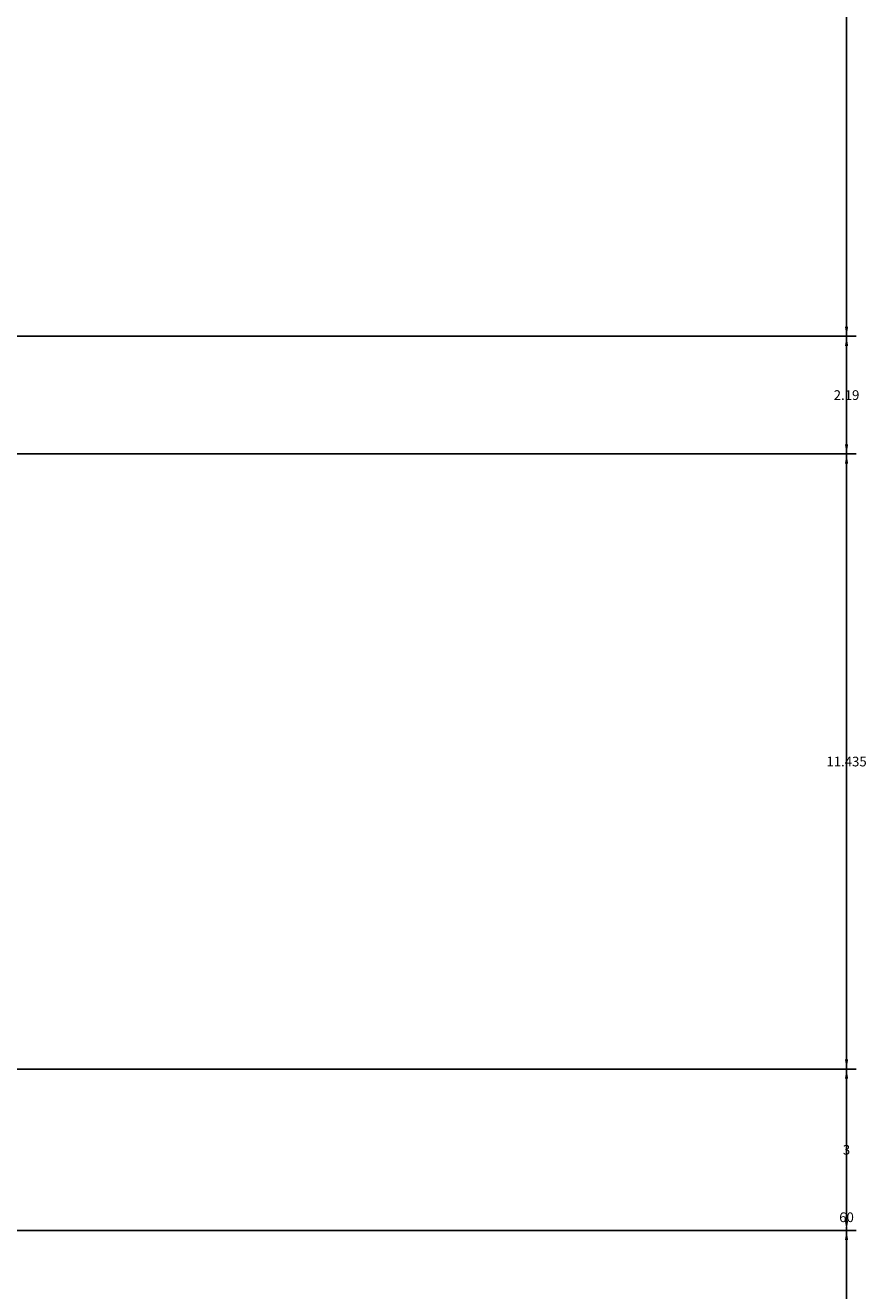
# Model space of a CAD drawing. Units: inches. Extents: x -6 to 289, y -8 to 323.
# Tile 105 of 107: x 273 to 289, y 276 to 299. Entities that reach past the tile are written whole.
import ezdxf

# ---------------------------------------------------------------- set-up
doc = ezdxf.new("R2010")
doc.units = ezdxf.units.IN
doc.header["$MEASUREMENT"] = 0
doc.layers.add('A-ANNO-DIMS', color=2, linetype='Continuous', lineweight=18)
doc.styles.get("Standard").update_dxf_attribs({"font": 'arial.ttf'})
doc.dimstyles.get("Standard").update_dxf_attribs({"dimtxt": 0.18, "dimasz": 0.18, "dimexe": 0.18, "dimexo": 0.0625, "dimgap": 0.09, "dimtad": 0, "dimtih": 1, "dimtoh": 1, "dimdec": 4, "dimzin": 0, "dimdsep": 46, "dimtxsty": 'Standard', "dimcen": 0.09, "dimadec": 0, "dimazin": 0, "dimtfac": 1, "dimtdec": 4, "dimtofl": 0, "dimtmove": 0, "dimatfit": 3, "dimfxl": 1, "dimtolj": 1, "dimtzin": 0, "dimarcsym": 0})

# ---------------------------------------------------------------- blocks, each defined once
blk = doc.blocks.new('*D27')
at = {"layer": 'A-ANNO-DIMS', "color": 0, "lineweight": -2, "transparency": 16777216}
for p, q in [((19.226, 307.289), (288.653, 307.289)), ((288.473, 307.109), (288.473, 277.471)), ((288.473, 247.469), (288.473, 277.107)), ((247.226, 247.289), (288.653, 247.289))]:
    blk.add_line(p, q, dxfattribs=at)
at = {"layer": 'A-ANNO-DIMS', "color": 0, "transparency": 16777216}
for points in [[(288.443, 307.109), (288.503, 307.109), (288.473, 307.289)], [(288.443, 247.469), (288.503, 247.469), (288.473, 247.289)]]:
    blk.add_solid(points, dxfattribs=at)
at = {"layer": 'Defpoints', "color": 0, "transparency": 16777216}
for p in [(19.164, 307.289), (288.473, 307.289), (247.164, 247.289)]:
    blk.add_point(p, dxfattribs=at)
at = {"layer": 'A-ANNO-DIMS', "color": 0, "transparency": 16777216, "insert": (288.473, 277.289), "char_height": 0.18, "attachment_point": 5}
blk.add_mtext('\\A1;60', dxfattribs=at)
blk = doc.blocks.new('*D114')
at = {"layer": 'A-ANNO-DIMS', "color": 0, "lineweight": -2, "transparency": 16777216}
for p, q in [((259.226, 277.043), (288.653, 277.043)), ((288.473, 276.863), (288.473, 268.348)), ((288.473, 259.469), (288.473, 267.984)), ((271.226, 259.289), (288.653, 259.289))]:
    blk.add_line(p, q, dxfattribs=at)
at = {"layer": 'A-ANNO-DIMS', "color": 0, "transparency": 16777216}
for points in [[(288.443, 276.863), (288.503, 276.863), (288.473, 277.043)], [(288.443, 259.469), (288.503, 259.469), (288.473, 259.289)]]:
    blk.add_solid(points, dxfattribs=at)
at = {"layer": 'Defpoints', "color": 0, "transparency": 16777216}
for p in [(259.164, 277.043), (288.473, 277.043), (271.164, 259.289)]:
    blk.add_point(p, dxfattribs=at)
at = {"layer": 'A-ANNO-DIMS', "color": 0, "transparency": 16777216, "insert": (288.473, 268.166), "char_height": 0.18, "attachment_point": 5}
blk.add_mtext('\\A1;17.754', dxfattribs=at)
blk = doc.blocks.new('*D115')
at = {"layer": 'A-ANNO-DIMS', "color": 0, "lineweight": -2, "transparency": 16777216}
for p, q in [((262.226, 280.043), (288.653, 280.043)), ((288.473, 279.863), (288.473, 278.725)), ((288.473, 277.223), (288.473, 278.361)), ((259.226, 277.043), (288.653, 277.043))]:
    blk.add_line(p, q, dxfattribs=at)
at = {"layer": 'A-ANNO-DIMS', "color": 0, "transparency": 16777216}
for points in [[(288.443, 279.863), (288.503, 279.863), (288.473, 280.043)], [(288.443, 277.223), (288.503, 277.223), (288.473, 277.043)]]:
    blk.add_solid(points, dxfattribs=at)
at = {"layer": 'Defpoints', "color": 0, "transparency": 16777216}
for p in [(262.164, 280.043), (288.473, 280.043), (259.164, 277.043)]:
    blk.add_point(p, dxfattribs=at)
at = {"layer": 'A-ANNO-DIMS', "color": 0, "transparency": 16777216, "insert": (288.473, 278.543), "char_height": 0.18, "attachment_point": 5}
blk.add_mtext('\\A1;3', dxfattribs=at)
blk = doc.blocks.new('*D116')
at = {"layer": 'A-ANNO-DIMS', "color": 0, "lineweight": -2, "transparency": 16777216}
for p, q in [((255.866, 291.478), (288.653, 291.478)), ((288.473, 291.298), (288.473, 285.942)), ((288.473, 280.223), (288.473, 285.578)), ((262.226, 280.043), (288.653, 280.043))]:
    blk.add_line(p, q, dxfattribs=at)
at = {"layer": 'A-ANNO-DIMS', "color": 0, "transparency": 16777216}
for points in [[(288.443, 291.298), (288.503, 291.298), (288.473, 291.478)], [(288.443, 280.223), (288.503, 280.223), (288.473, 280.043)]]:
    blk.add_solid(points, dxfattribs=at)
at = {"layer": 'Defpoints', "color": 0, "transparency": 16777216}
for p in [(255.804, 291.478), (288.473, 291.478), (262.164, 280.043)]:
    blk.add_point(p, dxfattribs=at)
at = {"layer": 'A-ANNO-DIMS', "color": 0, "transparency": 16777216, "insert": (288.473, 285.76), "char_height": 0.18, "attachment_point": 5}
blk.add_mtext('\\A1;11.435', dxfattribs=at)
blk = doc.blocks.new('*D117')
at = {"layer": 'A-ANNO-DIMS', "color": 0, "lineweight": -2, "transparency": 16777216}
for p, q in [((257.703, 293.666), (288.653, 293.666)), ((288.473, 293.486), (288.473, 292.754)), ((288.473, 291.658), (288.473, 292.39)), ((255.866, 291.478), (288.653, 291.478))]:
    blk.add_line(p, q, dxfattribs=at)
at = {"layer": 'A-ANNO-DIMS', "color": 0, "transparency": 16777216}
for points in [[(288.443, 293.486), (288.503, 293.486), (288.473, 293.666)], [(288.443, 291.658), (288.503, 291.658), (288.473, 291.478)]]:
    blk.add_solid(points, dxfattribs=at)
at = {"layer": 'Defpoints', "color": 0, "transparency": 16777216}
for p in [(257.641, 293.666), (288.473, 293.666), (255.804, 291.478)]:
    blk.add_point(p, dxfattribs=at)
at = {"layer": 'A-ANNO-DIMS', "color": 0, "transparency": 16777216, "insert": (288.473, 292.572), "char_height": 0.18, "attachment_point": 5}
blk.add_mtext('\\A1;2.19', dxfattribs=at)
blk = doc.blocks.new('*D118')
at = {"layer": 'A-ANNO-DIMS', "color": 0, "lineweight": -2, "transparency": 16777216}
for p, q in [((118.226, 307.289), (288.653, 307.289)), ((288.473, 307.109), (288.473, 300.659)), ((288.473, 293.846), (288.473, 300.295)), ((257.703, 293.666), (288.653, 293.666))]:
    blk.add_line(p, q, dxfattribs=at)
at = {"layer": 'A-ANNO-DIMS', "color": 0, "transparency": 16777216}
for points in [[(288.443, 307.109), (288.503, 307.109), (288.473, 307.289)], [(288.443, 293.846), (288.503, 293.846), (288.473, 293.666)]]:
    blk.add_solid(points, dxfattribs=at)
at = {"layer": 'Defpoints', "color": 0, "transparency": 16777216}
for p in [(118.164, 307.289), (288.473, 307.289), (257.641, 293.666)]:
    blk.add_point(p, dxfattribs=at)
at = {"layer": 'A-ANNO-DIMS', "color": 0, "transparency": 16777216, "insert": (288.473, 300.477), "char_height": 0.18, "attachment_point": 5}
blk.add_mtext('\\A1;13.623', dxfattribs=at)

msp = doc.modelspace()

# ---------------------------------------------------------------- dimensions: what is measured, and where the dimension line sits
at = {"layer": 'A-ANNO-DIMS'}
for base, p1, p2, override, picture, middle in [((288.4733, 307.2888), (247.1638, 247.2888), (19.1638, 307.2888), {"dimdec": 0, "dimlfac": 1, "dimrnd": 0, "dimzin": 0, "dimdsep": 46, "dimlunit": 2}, '*D27', (288.4733, 277.2888)), ((288.4733, 307.2888), (257.6407, 293.6657), (118.1638, 307.2888), {"dimdec": 3, "dimlfac": 1, "dimrnd": 0, "dimzin": 0, "dimdsep": 46, "dimlunit": 2}, '*D118', (288.4733, 300.4773)), ((288.4733, 293.6657), (255.8036, 291.4781), (257.6407, 293.6657), {"dimdec": 2, "dimlfac": 1, "dimrnd": 0, "dimzin": 0, "dimdsep": 46, "dimlunit": 2}, '*D117', (288.4733, 292.5719)), ((288.4733, 291.4781), (262.1638, 280.0427), (255.8036, 291.4781), {"dimdec": 3, "dimlfac": 1, "dimrnd": 0, "dimzin": 0, "dimdsep": 46, "dimlunit": 2}, '*D116', (288.4733, 285.7604)), ((288.4733, 280.0427), (259.1638, 277.0427), (262.1638, 280.0427), {"dimdec": 0, "dimlfac": 1, "dimrnd": 0, "dimzin": 0, "dimdsep": 46, "dimlunit": 2}, '*D115', (288.4733, 278.5427)), ((288.4733, 277.0427), (271.1638, 259.2888), (259.1638, 277.0427), {"dimdec": 3, "dimlfac": 1, "dimrnd": 0, "dimzin": 0, "dimdsep": 46, "dimlunit": 2}, '*D114', (288.4733, 268.1657))]:
    dim = msp.add_linear_dim(base=base, p1=p1, p2=p2, angle=90, dimstyle='Standard', override=override, dxfattribs=at)
    dim.commit()
    dim.dimension.update_dxf_attribs({"geometry": picture, "text_midpoint": middle})

doc.saveas('drawing.dxf')
